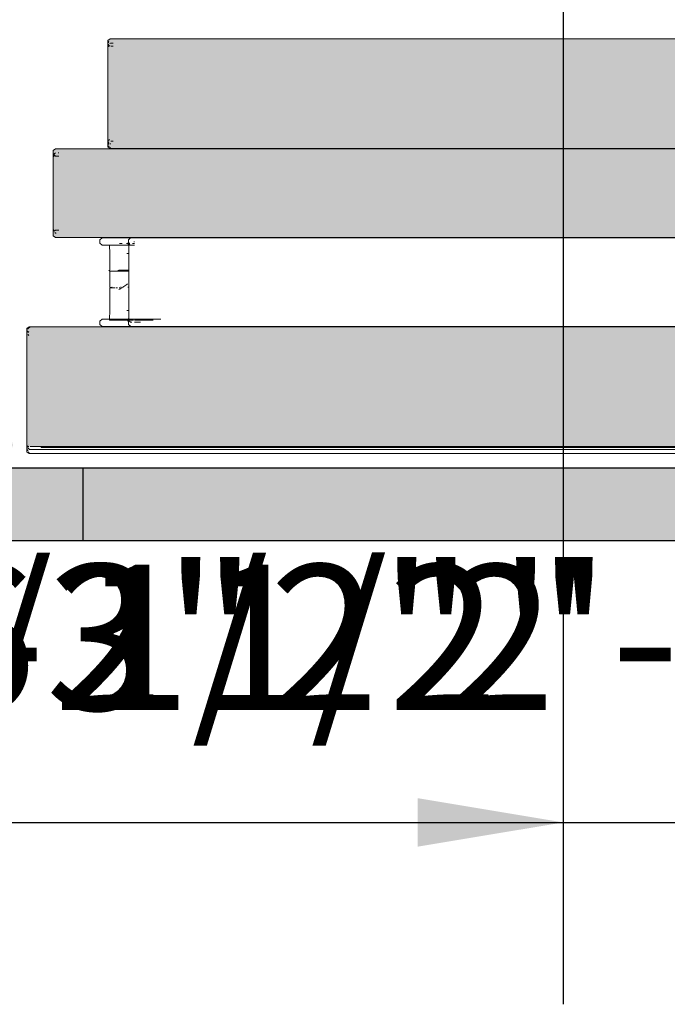
# Model space of a CAD drawing. Units: millimetres. Extents: x 7894 to 8038, y 6851 to 6951.
# Tile 17 of 49: x 7946.604 to 7951.055, y 6903.287 to 6910.053. Entities that reach past the tile are written whole.
import ezdxf

# ---------------------------------------------------------------- set-up
doc = ezdxf.new("R2010")
doc.units = ezdxf.units.MM
for name, color, linetype, lineweight in [('A-ANNO-DIMS', 2, 'Continuous', 18), ('A-FURN-BOOK', 8, 'Continuous', 13), ('A-FURN-SHLF', 7, 'Continuous', 30)]:
    doc.layers.add(name, color=color, linetype=linetype, lineweight=lineweight)
doc.layers.add('A-FURN-PATT', color=32, linetype='Continuous', lineweight=9, true_color=0xcd6928)
doc.styles.get("Standard").update_dxf_attribs({"font": 'arial.ttf'})
doc.dimstyles.new('ISO-25', dxfattribs={"dimtxt": 1, "dimasz": 1, "dimexe": 1.25, "dimexo": 0.625, "dimtad": 1, "dimdec": 0, "dimlunit": 4, "dimtxsty": 'Standard', "dimcen": 2.5, "dimclrt": 1, "dimadec": 0, "dimazin": 0, "dimtfac": 1, "dimtdec": 0, "dimtmove": 0, "dimatfit": 3, "dimfxl": 1, "dimarcsym": 0})

# ---------------------------------------------------------------- blocks, each defined once
blk = doc.blocks.new('*D23')
at = {"layer": 'A-ANNO-DIMS', "color": 0, "lineweight": -2, "transparency": 16777216}
for p, q in [((7940.0888, 6907.098), (7940.0888, 6947.7928)), ((7971.9356, 6928.989), (7971.9356, 6947.7928)), ((7941.0888, 6946.5428), (7970.9356, 6946.5428))]:
    blk.add_line(p, q, dxfattribs=at)
at = {"layer": 'A-ANNO-DIMS', "color": 0, "transparency": 16777216}
for points in [[(7941.0888, 6946.7095), (7941.0888, 6946.3762), (7940.0888, 6946.5428)], [(7970.9356, 6946.7095), (7970.9356, 6946.3762), (7971.9356, 6946.5428)]]:
    blk.add_solid(points, dxfattribs=at)
at = {"layer": 'Defpoints', "color": 0, "transparency": 16777216}
for p in [(7971.9356, 6946.5428), (7971.9356, 6928.364), (7940.0888, 6906.473)]:
    blk.add_point(p, dxfattribs=at)
at = {"layer": 'A-ANNO-DIMS', "color": 1, "transparency": 16777216, "insert": (7956.0122, 6947.6784), "char_height": 1, "attachment_point": 5}
blk.add_mtext('2\'-8"', dxfattribs=at)
blk = doc.blocks.new('*D24')
at = {"layer": 'A-ANNO-DIMS', "color": 0, "lineweight": -2, "transparency": 16777216}
for p, q in [((7953.3408, 6944.6059), (7936.9023, 6944.6059)), ((7938.1523, 6907.473), (7938.1523, 6943.6059)), ((7939.4638, 6906.473), (7936.9023, 6906.473))]:
    blk.add_line(p, q, dxfattribs=at)
at = {"layer": 'A-ANNO-DIMS', "color": 0, "transparency": 16777216}
for points in [[(7937.9856, 6943.6059), (7938.319, 6943.6059), (7938.1523, 6944.6059)], [(7937.9856, 6907.473), (7938.319, 6907.473), (7938.1523, 6906.473)]]:
    blk.add_solid(points, dxfattribs=at)
at = {"layer": 'Defpoints', "color": 0, "transparency": 16777216}
for p in [(7938.1523, 6944.6059), (7953.9658, 6944.6059), (7940.0888, 6906.473)]:
    blk.add_point(p, dxfattribs=at)
at = {"layer": 'A-ANNO-DIMS', "color": 1, "transparency": 16777216, "insert": (7937.0164, 6925.5395), "char_height": 1, "attachment_point": 5, "rotation": 90}
blk.add_mtext('3\'-2"', dxfattribs=at)
blk = doc.blocks.new('*D25')
at = {"layer": 'A-ANNO-DIMS', "color": 0, "lineweight": -2, "transparency": 16777216}
for p, q in [((7940.0888, 6905.848), (7940.0888, 6903.2865)), ((7964.3408, 6905.8484), (7964.3408, 6903.2865)), ((7941.0888, 6904.5365), (7963.3408, 6904.5365))]:
    blk.add_line(p, q, dxfattribs=at)
at = {"layer": 'A-ANNO-DIMS', "color": 0, "transparency": 16777216}
for points in [[(7941.0888, 6904.7032), (7941.0888, 6904.3699), (7940.0888, 6904.5365)], [(7963.3408, 6904.7032), (7963.3408, 6904.3699), (7964.3408, 6904.5365)]]:
    blk.add_solid(points, dxfattribs=at)
at = {"layer": 'Defpoints', "color": 0, "transparency": 16777216}
for p in [(7940.0888, 6906.473), (7964.3408, 6906.4734), (7964.3408, 6904.5365)]:
    blk.add_point(p, dxfattribs=at)
at = {"layer": 'A-ANNO-DIMS', "color": 1, "transparency": 16777216, "insert": (7952.2148, 6905.6786), "char_height": 1, "attachment_point": 5}
blk.add_mtext('2\'-0 1/2"', dxfattribs=at)
blk = doc.blocks.new('*D26')
at = {"layer": 'A-ANNO-DIMS', "color": 0, "lineweight": -2, "transparency": 16777216}
for p, q in [((7950.9654, 6918.7198), (7975.2272, 6918.7198)), ((7973.9772, 6917.7198), (7973.9772, 6907.4734)), ((7964.9658, 6906.4734), (7975.2272, 6906.4734))]:
    blk.add_line(p, q, dxfattribs=at)
at = {"layer": 'A-ANNO-DIMS', "color": 0, "transparency": 16777216}
for points in [[(7973.8105, 6917.7198), (7974.1439, 6917.7198), (7973.9772, 6918.7198)], [(7973.8105, 6907.4734), (7974.1439, 6907.4734), (7973.9772, 6906.4734)]]:
    blk.add_solid(points, dxfattribs=at)
at = {"layer": 'Defpoints', "color": 0, "transparency": 16777216}
for p in [(7950.3404, 6918.7198), (7964.3408, 6906.4734), (7973.9772, 6906.4734)]:
    blk.add_point(p, dxfattribs=at)
at = {"layer": 'A-ANNO-DIMS', "color": 1, "transparency": 16777216, "insert": (7972.8416, 6912.5966), "char_height": 1, "attachment_point": 5, "rotation": 90}
blk.add_mtext('1\'-0"', dxfattribs=at)
blk = doc.blocks.new('*D29')
at = {"layer": 'A-ANNO-DIMS', "color": 0, "lineweight": -2, "transparency": 16777216}
for p, q in [((7940.4346, 6923.8139), (7940.4346, 6903.2865)), ((7943.7365, 6918.0948), (7943.7365, 6903.2865)), ((7941.4346, 6904.5365), (7942.7365, 6904.5365)), ((7943.7365, 6904.5365), (7950.9749, 6904.5365))]:
    blk.add_line(p, q, dxfattribs=at)
at = {"layer": 'A-ANNO-DIMS', "color": 0, "transparency": 16777216}
for points in [[(7941.4346, 6904.7032), (7941.4346, 6904.3699), (7940.4346, 6904.5365)], [(7942.7365, 6904.7032), (7942.7365, 6904.3699), (7943.7365, 6904.5365)]]:
    blk.add_solid(points, dxfattribs=at)
at = {"layer": 'Defpoints', "color": 0, "transparency": 16777216}
for p in [(7940.4346, 6924.4389), (7943.7365, 6918.7198), (7943.7365, 6904.5365)]:
    blk.add_point(p, dxfattribs=at)
at = {"layer": 'A-ANNO-DIMS', "color": 1, "transparency": 16777216, "insert": (7947.8557, 6905.6789), "char_height": 1, "attachment_point": 5}
blk.add_mtext('0\'-3 1/2"', dxfattribs=at)
blk = doc.blocks.new('*D32')
at = {"layer": 'A-ANNO-DIMS', "color": 0, "lineweight": -2, "transparency": 16777216}
for p, q in [((7943.7365, 6918.0948), (7943.7365, 6903.2865)), ((7950.3404, 6918.0948), (7950.3404, 6903.2865)), ((7944.7365, 6904.5365), (7949.3404, 6904.5365))]:
    blk.add_line(p, q, dxfattribs=at)
at = {"layer": 'A-ANNO-DIMS', "color": 0, "transparency": 16777216}
for points in [[(7944.7365, 6904.7032), (7944.7365, 6904.3699), (7943.7365, 6904.5365)], [(7949.3404, 6904.7032), (7949.3404, 6904.3699), (7950.3404, 6904.5365)]]:
    blk.add_solid(points, dxfattribs=at)
at = {"layer": 'Defpoints', "color": 0, "transparency": 16777216}
for p in [(7943.7365, 6918.7198), (7950.3404, 6918.7198), (7950.3404, 6904.5365)]:
    blk.add_point(p, dxfattribs=at)
at = {"layer": 'A-ANNO-DIMS', "color": 1, "transparency": 16777216, "insert": (7947.0385, 6905.6786), "char_height": 1, "attachment_point": 5}
blk.add_mtext('0\'-6 1/2"', dxfattribs=at)
blk = doc.blocks.new('*D33')
at = {"layer": 'A-ANNO-DIMS', "color": 0, "lineweight": -2, "transparency": 16777216}
for p, q in [((7940.4346, 6923.8139), (7940.4346, 6903.2865)), ((7940.0888, 6905.848), (7940.0888, 6903.2865)), ((7939.0888, 6904.5365), (7938.0888, 6904.5365)), ((7940.0888, 6904.5365), (7940.4346, 6904.5365)), ((7941.4346, 6904.5365), (7948.673, 6904.5365))]:
    blk.add_line(p, q, dxfattribs=at)
at = {"layer": 'A-ANNO-DIMS', "color": 0, "transparency": 16777216}
for points in [[(7939.0888, 6904.7032), (7939.0888, 6904.3699), (7940.0888, 6904.5365)], [(7941.4346, 6904.7032), (7941.4346, 6904.3699), (7940.4346, 6904.5365)]]:
    blk.add_solid(points, dxfattribs=at)
at = {"layer": 'Defpoints', "color": 0, "transparency": 16777216}
for p in [(7940.4346, 6924.4389), (7940.0888, 6906.473), (7940.4346, 6904.5365)]:
    blk.add_point(p, dxfattribs=at)
at = {"layer": 'A-ANNO-DIMS', "color": 1, "transparency": 16777216, "insert": (7945.5538, 6905.6786), "char_height": 1, "attachment_point": 5}
blk.add_mtext('0\'-0 1/2"', dxfattribs=at)

msp = doc.modelspace()

# ---------------------------------------------------------------- hatches: boundary and pattern name
at = {"layer": 'A-FURN-PATT'}
h = msp.add_hatch(color=256, dxfattribs=at)
h.dxf.hatch_style = 1
h.paths.add_polyline_path([(7942.8406, 6913.3629), (7942.8593, 6913.356), (7942.8677, 6913.356), (7942.8677, 6914.2132), (7942.876, 6914.2376), (7942.8813, 6914.2376), (7942.9022, 6914.2457), (7943.3657, 6914.2457), (7943.3844, 6914.2376), (7943.3861, 6914.2376), (7943.3858, 6914.2132), (7943.3852, 6913.2312), (7943.3944, 6906.9948), (7943.387, 6906.9732), (7943.4027, 6906.9732), (7943.403, 6906.9948), (7943.4029, 6908.4372), (7943.3944, 6914.2132), (7943.4169, 6914.2376), (7943.4198, 6914.2457), (7943.4555, 6914.2457), (7943.4603, 6914.238), (7943.8607, 6914.2452), (7943.8615, 6914.2457), (7943.8623, 6914.2452), (7943.8866, 6914.2457), (7943.8944, 6914.2402), (7943.9104, 6914.2376), (7943.9211, 6914.2132), (7943.9294, 6914.2376), (7943.9318, 6914.2376), (7943.9453, 6914.2398), (7943.9488, 6914.2457), (7943.9797, 6914.2452), (7943.9807, 6914.2457), (7943.9815, 6914.2451), (7944.3738, 6914.2376), (7944.3882, 6914.2457), (7944.4201, 6914.2457), (7944.4341, 6914.2376), (7944.4395, 6914.2376), (7944.4478, 6914.2132), (7944.4478, 6914.1031), (7944.4622, 6914.099), (7944.7359, 6914.1607), (7944.8923, 6914.2014), (7944.9541, 6914.2098), (7944.955, 6914.21), (7946.556, 6907.1325), (7946.5534, 6907.1122), (7946.5529, 6907.1152), (7946.499, 6907.103), (7946.3343, 6907.0604), (7946.0282, 6906.9914), (7945.6731, 6908.5712), (7944.4484, 6914.0015), (7944.4478, 6906.9948), (7944.4404, 6906.9732), (7947.0373, 6906.9734), (7964.3408, 6906.9734), (7964.3408, 6906.4734), (7947.0373, 6906.4734), (7940.0888, 6906.473), (7940.0888, 6906.973), (7941.9951, 6906.9731), (7941.9899, 6906.9898), (7941.9899, 6913.3353), (7941.9968, 6913.3574), (7942.003, 6913.3571), (7942.0169, 6913.3629), (7942.0366, 6913.3629), (7942.0378, 6913.3629), (7942.0479, 6913.356), (7942.8142, 6913.356), (7942.8157, 6913.356), (7942.8346, 6913.356)])
h.paths.add_polyline_path([(7942.8598, 6913.0201), (7942.861, 6913.3353), (7942.8677, 6906.9948), (7942.876, 6906.9759), (7942.876, 6906.9903), (7942.8813, 6914.2376), (7942.876, 6914.2321), (7942.876, 6914.2177), (7942.8809, 6906.9647), (7942.8784, 6906.9704), (7942.876, 6906.9704), (7942.8574, 6906.9704), (7942.8613, 6911.8549)], flags=16)
h.paths.add_polyline_path([(7942.8613, 6911.8549), (7942.8677, 6906.9948), (7942.8686, 6906.9921), (7942.8677, 6906.9898), (7942.8616, 6906.9704), (7942.8598, 6906.9704), (7942.8574, 6906.9704), (7942.0002, 6906.9704), (7941.9978, 6906.9704), (7941.996, 6906.9704), (7941.9899, 6906.9898), (7941.9978, 6906.9704), (7942.0002, 6906.9704), (7942.8598, 6906.9704), (7942.8616, 6906.9748)], flags=16)
h.paths.add_polyline_path([(7942.023, 6913.356), (7942.0169, 6913.3629), (7942.0366, 6913.3629), (7942.0378, 6913.3629), (7942.0367, 6913.3614), (7942.0369, 6913.356)], flags=16)
h.paths.add_polyline_path([(7942.0366, 6913.3629), (7942.0169, 6913.3629), (7942.0196, 6913.3598)], flags=0)
h.paths.add_polyline_path([(7942.0353, 6913.356), (7942.0369, 6913.356), (7942.0367, 6913.3614)], flags=0)
h.paths.add_polyline_path([(7943.9293, 6906.9759), (7943.9211, 6906.9948), (7943.9294, 6906.9704)], flags=0)
h.paths.add_polyline_path([(7943.9125, 6914.2132), (7943.8982, 6914.2376), (7943.8944, 6914.2402), (7943.8832, 6914.2421), (7943.8781, 6914.2367), (7943.8765, 6914.2376), (7943.8789, 6914.2376), (7943.8866, 6914.2457), (7943.8623, 6914.2452), (7943.8607, 6914.2452), (7943.8615, 6914.2457), (7943.8623, 6914.2452), (7943.8866, 6914.2457), (7943.8944, 6914.2402), (7943.8982, 6914.2376), (7943.9097, 6914.218), (7943.9125, 6914.2168), (7943.9079, 6906.9704), (7943.9104, 6906.9704), (7943.9211, 6914.2132), (7943.9294, 6914.2376), (7943.9318, 6914.2376), (7943.9453, 6914.2398), (7943.9488, 6914.2457), (7943.9797, 6914.2452), (7943.9807, 6914.2457), (7943.9815, 6914.2451), (7944.3738, 6914.2376), (7944.3882, 6914.2457), (7944.4201, 6914.2457), (7944.4341, 6914.2376), (7944.4395, 6914.2376), (7944.4395, 6914.2177), (7944.4341, 6914.0941), (7944.4478, 6914.1004), (7944.4513, 6914.1021), (7944.4622, 6914.099), (7944.4343, 6914.0927), (7944.429, 6914.0915), (7944.4341, 6914.069), (7944.4484, 6914.0015), (7944.4341, 6914.0649), (7944.4346, 6906.9704), (7944.4371, 6906.9704), (7944.4395, 6906.9759), (7944.4395, 6906.9704), (7943.931, 6906.9704), (7943.9128, 6906.9704), (7943.9079, 6906.9704)], flags=16)
h.paths.add_polyline_path([(7943.9211, 6914.2132), (7943.9294, 6914.2376), (7943.9318, 6914.2376), (7943.9453, 6914.2398), (7943.9488, 6914.2457), (7943.9797, 6914.2452), (7943.9807, 6914.2457), (7943.9815, 6914.2451), (7944.3738, 6914.2376), (7944.3882, 6914.2457), (7944.4201, 6914.2457), (7944.4321, 6914.2387), (7944.4249, 6914.2376), (7944.4041, 6914.2376), (7944.4032, 6914.2136), (7944.4032, 6914.2376), (7944.4025, 6914.2379), (7944.3897, 6914.2382), (7944.3753, 6914.2384), (7944.3738, 6914.2376), (7943.9815, 6914.2451), (7943.9488, 6914.2457), (7943.9453, 6914.2398), (7943.9294, 6914.2132), (7943.931, 6906.9721), (7943.931, 6906.9704), (7943.9294, 6906.9704), (7943.9293, 6906.9759), (7943.9294, 6914.2132), (7943.9439, 6914.2376), (7943.9318, 6914.2376)], flags=0)
h.paths.add_polyline_path([(7942.8813, 6914.2376), (7942.8778, 6914.2362), (7942.8796, 6914.2404), (7942.885, 6914.239)], flags=17)
h.paths.add_polyline_path([(7944.4116, 6914.242), (7944.4104, 6914.2408), (7944.4125, 6914.2418)], flags=0)
h.paths.add_polyline_path([(7944.3879, 6914.2382), (7944.3882, 6914.2457), (7944.4094, 6914.241), (7944.4103, 6914.2408), (7944.4036, 6914.2373), (7944.39, 6914.2447), (7944.3897, 6914.2382)], flags=0)
h.paths.add_polyline_path([(7963.1359, 6906.9526), (7963.1396, 6906.9526), (7963.1431, 6906.9582)], flags=16)
h.paths.add_polyline_path([(7954.3975, 6907.3902), (7954.397, 6907.3948), (7954.3984, 6907.4007), (7954.3975, 6907.567), (7954.3984, 6907.5978), (7954.3986, 6907.7694), (7954.3978, 6907.7989), (7954.399, 6907.8759), (7954.3992, 6907.9037), (7954.3944, 6907.9081), (7954.4019, 6907.9055), (7954.3996, 6907.93), (7954.3988, 6907.9307), (7954.3841, 6907.9429), (7946.6754, 6907.9429), (7946.6535, 6907.9232), (7946.6531, 6907.9127), (7946.6527, 6907.7694), (7946.6525, 6907.4007), (7946.653, 6907.1185), (7946.6574, 6907.1224), (7946.656, 6907.1145), (7946.6571, 6907.1135), (7946.6675, 6907.1209), (7946.7515, 6907.1209), (7946.9105, 6907.1209), (7954.3003, 6907.1209), (7954.3895, 6907.1209), (7954.3915, 6907.1191), (7954.3991, 6907.1209), (7954.399, 6907.1383), (7954.3978, 6907.2163), (7954.3986, 6907.2413)], flags=17)
h.paths.add_polyline_path([(7954.3003, 6907.1209), (7954.3003, 6907.1136), (7946.9105, 6907.1129), (7946.7516, 6907.1136), (7946.7515, 6907.1209), (7946.6675, 6907.1209), (7946.6531, 6907.1106), (7946.653, 6907.1185), (7946.6574, 6907.1224), (7946.656, 6907.1145), (7946.6571, 6907.1135), (7946.6675, 6907.1209), (7946.7515, 6907.1209), (7946.9105, 6907.1209)], flags=17)
h.paths.add_polyline_path([(7954.3981, 6907.9048), (7954.3944, 6907.9081), (7954.3997, 6907.9062), (7954.4007, 6907.9186), (7954.4019, 6907.9055), (7954.405, 6907.9072), (7954.4044, 6907.9046), (7954.4027, 6907.8974), (7954.4024, 6907.9009), (7954.3996, 6907.9034), (7954.3996, 6907.9025), (7954.3994, 6907.9023), (7954.3995, 6907.9035)], flags=17)
h = msp.add_hatch(color=256, dxfattribs=at)
h.dxf.hatch_style = 1
h.paths.add_polyline_path([(7954.384, 6909.6263), (7954.383, 6909.6719), (7954.3832, 6909.6719), (7954.3841, 6909.7804), (7954.3842, 6909.8528), (7954.3843, 6909.8691), (7954.3797, 6909.8762), (7954.3846, 6909.8799), (7954.3847, 6909.8812), (7954.3833, 6909.8825), (7954.3848, 6909.8826), (7954.3858, 6909.8967), (7954.3849, 6909.9082), (7954.384, 6909.909), (7954.384, 6909.9101), (7954.3682, 6909.9217), (7947.2251, 6909.9217), (7947.21, 6909.9101), (7947.2092, 6909.8906), (7947.2092, 6909.1993), (7947.2105, 6909.1985), (7947.2109, 6909.2125), (7947.2127, 6909.2113), (7947.2135, 6909.2114), (7947.2139, 6909.2117), (7947.2148, 6909.196), (7947.2105, 6909.1985), (7947.21, 6909.1798), (7947.2251, 6909.1682), (7947.2316, 6909.1682), (7954.3693, 6909.1682), (7954.384, 6909.1798), (7954.385, 6909.1814), (7954.3858, 6909.1921), (7954.3871, 6909.207), (7954.3814, 6909.2115), (7954.377, 6909.2116), (7954.3506, 6909.2116), (7954.3427, 6909.2213), (7954.373, 6909.2213), (7954.3747, 6909.2192), (7954.3833, 6909.2192), (7954.3833, 6909.2247), (7954.3843, 6909.2237), (7954.3842, 6909.2371), (7954.384, 6909.4541), (7954.3827, 6909.477), (7954.3832, 6909.477)])
h.paths.add_polyline_path([(7947.2139, 6909.8782), (7947.214, 6909.8795), (7947.2135, 6909.8785)], flags=16)
h.paths.add_polyline_path([(7947.2105, 6909.1985), (7947.2109, 6909.2125), (7947.2127, 6909.2113), (7947.2135, 6909.2114), (7947.2139, 6909.2117), (7947.2144, 6909.2034), (7947.2148, 6909.196)], flags=17)
h.paths.add_polyline_path([(7954.3858, 6909.1921), (7954.3848, 6909.2088), (7954.3871, 6909.207)], flags=17)
h.paths.add_polyline_path([(7954.5846, 6909.1237), (7954.5837, 6909.1245), (7954.5808, 6909.1271), (7954.5846, 6909.1307), (7954.5846, 6909.1519), (7954.5691, 6909.1658), (7946.8503, 6909.1658), (7946.8349, 6909.1546), (7946.8349, 6909.1307), (7946.8349, 6909.1147), (7946.8349, 6909.1147), (7946.8349, 6908.5685), (7946.8503, 6908.5572), (7954.5691, 6908.5572), (7954.5846, 6908.5685)])
h.paths.add_polyline_path([(7946.8375, 6909.1282), (7946.8349, 6909.1263), (7946.8349, 6909.1237), (7946.8473, 6909.1162), (7946.8503, 6909.1162)], flags=16)

# ---------------------------------------------------------------- linework, layer by layer
at = {"layer": 'A-FURN-BOOK'}
for p, q in [((7947.2092, 6909.8906), (7947.21, 6909.9101)), ((7947.2092, 6909.8906), (7947.2092, 6909.1993)), ((7947.21, 6909.9101), (7947.2251, 6909.9217)), ((7947.21, 6909.9101), (7947.2105, 6909.8913)), ((7947.2106, 6909.8888), (7947.2113, 6909.8799)), ((7947.2119, 6909.8784), (7947.2113, 6909.8799)), ((7947.2119, 6909.8784), (7947.2135, 6909.8785)), ((7947.2131, 6909.8717), (7947.2119, 6909.8784)), ((7947.2135, 6909.8785), (7947.214, 6909.8795)), ((7947.2135, 6909.8785), (7947.2227, 6909.8701)), ((7947.214, 6909.8795), (7947.2142, 6909.8839)), ((7947.2164, 6909.8811), (7947.214, 6909.8795)), ((7947.2148, 6909.8938), (7947.2153, 6909.901)), ((7947.2153, 6909.901), (7947.2159, 6909.9056)), ((7947.229, 6909.8928), (7947.2242, 6909.8884)), ((7954.3693, 6909.9217), (7947.2251, 6909.9217)), ((7947.2472, 6909.8928), (7947.229, 6909.8928)), ((7947.2135, 6909.8692), (7947.2131, 6909.8717)), ((7947.2156, 6909.8672), (7947.2135, 6909.8692)), ((7947.2242, 6909.8703), (7947.2227, 6909.8701)), ((7947.2316, 6909.8707), (7947.2471, 6909.8707)), ((7947.2105, 6909.1985), (7947.2092, 6909.1993)), ((7947.21, 6909.1798), (7947.2105, 6909.1985)), ((7947.2105, 6909.1985), (7947.2108, 6909.2098)), ((7947.2108, 6909.2098), (7947.2114, 6909.2111)), ((7947.2114, 6909.2111), (7947.212, 6909.2127)), ((7947.2135, 6909.2114), (7947.2114, 6909.2111)), ((7947.212, 6909.2127), (7947.2128, 6909.217)), ((7947.2147, 6909.2126), (7947.2135, 6909.2114)), ((7947.214, 6909.2104), (7947.2135, 6909.2114)), ((7947.2144, 6909.2034), (7947.214, 6909.2104)), ((7947.2164, 6909.2087), (7947.214, 6909.2104)), ((7947.2148, 6909.196), (7947.2144, 6909.2034)), ((7947.2226, 6909.2291), (7947.2156, 6909.2227)), ((7947.229, 6909.1971), (7947.2242, 6909.2015)), ((7947.2471, 6909.2192), (7947.2316, 6909.2192)), ((7946.8349, 6909.1546), (7946.8503, 6909.1658)), ((7946.8349, 6909.1307), (7946.8349, 6909.1546)), ((7946.8503, 6909.1377), (7946.8349, 6909.1263)), ((7946.8349, 6909.1263), (7946.8349, 6909.1307)), ((7946.8503, 6909.1162), (7946.8349, 6909.1307)), ((7954.5691, 6909.1658), (7946.8503, 6909.1658)), ((7946.8732, 6909.1377), (7946.868, 6909.1377)), ((7947.2251, 6909.1682), (7947.21, 6909.1798)), ((7947.2161, 6909.1825), (7947.2155, 6909.1869)), ((7947.2193, 6909.1795), (7947.2161, 6909.1825)), ((7947.2316, 6909.1682), (7947.2249, 6909.1744)), ((7947.2251, 6909.1682), (7947.2316, 6909.1682)), ((7947.2316, 6909.1682), (7954.3693, 6909.1682)), ((7946.8349, 6909.1237), (7946.8349, 6909.1263)), ((7946.8484, 6909.1155), (7946.8349, 6909.1237)), ((7946.8349, 6909.1147), (7946.8349, 6909.1237)), ((7946.8383, 6909.1116), (7946.8349, 6909.1147)), ((7946.8349, 6908.5685), (7946.8349, 6909.1147)), ((7946.8732, 6909.1162), (7946.8503, 6909.1162)), ((7946.8383, 6908.6114), (7946.8363, 6908.6096)), ((7946.8484, 6908.6075), (7946.84, 6908.6014)), ((7946.8413, 6908.5987), (7946.8503, 6908.6068)), ((7946.8503, 6908.5853), (7946.8454, 6908.5898)), ((7946.8503, 6908.6068), (7946.8732, 6908.6068)), ((7946.8503, 6908.5572), (7946.8349, 6908.5685)), ((7946.8555, 6908.5853), (7946.8503, 6908.5853)), ((7954.5691, 6908.5572), (7946.8503, 6908.5572)), ((7947.1561, 6908.5403), (7947.1715, 6908.5542)), ((7947.1561, 6908.5185), (7947.1561, 6908.5403)), ((7947.3682, 6908.5542), (7947.1715, 6908.5542)), ((7947.3517, 6908.5299), (7947.3504, 6908.5168)), ((7947.3526, 6908.5411), (7947.3517, 6908.5299)), ((7947.3517, 6908.5299), (7947.3528, 6908.516)), ((7947.3535, 6908.543), (7947.3526, 6908.5411)), ((7947.3536, 6908.5419), (7947.3526, 6908.5411)), ((7947.3535, 6908.543), (7947.3623, 6908.5492)), ((7947.3623, 6908.5492), (7947.3543, 6908.5425)), ((7947.3682, 6908.5542), (7947.3623, 6908.5492)), ((7947.3682, 6908.5542), (7954.5763, 6908.5542)), ((7947.3931, 6908.5261), (7947.3883, 6908.5261)), ((7947.1715, 6908.5046), (7947.1561, 6908.5185)), ((7947.1715, 6908.5046), (7947.2224, 6908.5046)), ((7947.223, 6908.4455), (7947.2224, 6908.5046)), ((7947.344, 6908.5046), (7947.2224, 6908.5046)), ((7947.2904, 6908.516), (7947.2891, 6908.5158)), ((7947.2904, 6908.516), (7947.3087, 6908.5158)), ((7947.3387, 6908.516), (7947.3479, 6908.516)), ((7947.344, 6908.5046), (7947.3495, 6908.5038)), ((7947.3474, 6908.5185), (7947.3479, 6908.516)), ((7947.3504, 6908.5168), (7947.3474, 6908.5185)), ((7947.3479, 6908.516), (7947.3504, 6908.5168)), ((7947.3479, 6908.516), (7947.3482, 6908.5147)), ((7947.3482, 6908.5147), (7947.3491, 6908.5074)), ((7947.3491, 6908.5074), (7947.3495, 6908.5038)), ((7947.3495, 6908.5038), (7947.35, 6908.5031)), ((7947.3495, 6908.5038), (7947.3532, 6908.5031)), ((7947.3504, 6908.5168), (7947.35, 6908.5122)), ((7947.3527, 6908.5138), (7947.35, 6908.5122)), ((7947.3533, 6908.5002), (7947.35, 6908.5031)), ((7947.3504, 6908.5168), (7947.3528, 6908.516)), ((7947.3542, 6908.516), (7947.3527, 6908.5147)), ((7947.3528, 6908.516), (7947.3527, 6908.5147)), ((7947.3527, 6908.5147), (7947.3527, 6908.5138)), ((7947.365, 6908.5046), (7947.3527, 6908.5138)), ((7947.3628, 6908.5046), (7947.3527, 6908.5138)), ((7947.3527, 6908.5138), (7947.3532, 6908.5031)), ((7947.3528, 6908.516), (7947.3542, 6908.516)), ((7947.3579, 6908.5046), (7947.3532, 6908.5031)), ((7947.3532, 6908.5031), (7947.3668, 6908.5033)), ((7947.3532, 6908.5031), (7947.3533, 6908.5002)), ((7947.3533, 6908.5002), (7947.3534, 6908.4872)), ((7947.3547, 6908.4988), (7947.3533, 6908.5002)), ((7947.3534, 6908.4872), (7947.3546, 6908.4455)), ((7947.358, 6908.5195), (7947.3542, 6908.516)), ((7947.3542, 6908.516), (7947.3608, 6908.516)), ((7947.3628, 6908.5046), (7947.3579, 6908.5046)), ((7947.365, 6908.5046), (7947.3628, 6908.5046)), ((7947.3668, 6908.5033), (7947.365, 6908.5046)), ((7947.3703, 6908.5046), (7947.365, 6908.5046)), ((7947.3668, 6908.5033), (7947.3703, 6908.5046)), ((7947.3932, 6908.5046), (7947.3703, 6908.5046)), ((7947.3797, 6908.516), (7947.3931, 6908.516)), ((7947.2236, 6908.3704), (7947.223, 6908.4455)), ((7947.3546, 6908.4455), (7947.3402, 6908.4455)), ((7947.3546, 6908.4455), (7947.3538, 6908.4287)), ((7947.3538, 6908.4287), (7947.3539, 6908.3323)), ((7947.2237, 6908.3323), (7947.2168, 6908.3291)), ((7947.2238, 6908.3258), (7947.2168, 6908.3291)), ((7947.2236, 6908.3704), (7947.2237, 6908.3323)), ((7947.2239, 6908.2877), (7947.2238, 6908.3258)), ((7947.2238, 6908.3258), (7947.3539, 6908.3258)), ((7947.2778, 6908.3291), (7947.2844, 6908.3291)), ((7947.3539, 6908.3323), (7947.285, 6908.3323)), ((7947.3275, 6908.3291), (7947.3539, 6908.3291)), ((7947.3548, 6908.3323), (7947.3539, 6908.3323)), ((7947.3539, 6908.3323), (7947.3539, 6908.3291)), ((7947.3539, 6908.3291), (7947.3548, 6908.3291)), ((7947.3539, 6908.3291), (7947.3539, 6908.3258)), ((7947.3539, 6908.3258), (7947.3548, 6908.3258)), ((7947.3539, 6908.3258), (7947.354, 6908.3136)), ((7947.2239, 6908.2877), (7947.2239, 6908.2159)), ((7947.354, 6908.3136), (7947.354, 6908.2159)), ((7947.2239, 6908.2093), (7947.2236, 6908.1299)), ((7947.2346, 6908.2126), (7947.2239, 6908.2159)), ((7947.2239, 6908.2093), (7947.2346, 6908.2126)), ((7947.2586, 6908.2093), (7947.2239, 6908.2093)), ((7947.2372, 6908.2159), (7947.2409, 6908.2159)), ((7947.2756, 6908.2093), (7947.2643, 6908.2093)), ((7947.2846, 6908.1978), (7947.2926, 6908.2011)), ((7947.2921, 6908.2093), (7947.2872, 6908.2093)), ((7947.3045, 6908.2093), (7947.2926, 6908.2011)), ((7947.2972, 6908.2159), (7947.3021, 6908.2159)), ((7947.3045, 6908.2093), (7947.314, 6908.2159)), ((7947.3075, 6908.2093), (7947.3045, 6908.2093)), ((7947.314, 6908.2159), (7947.3395, 6908.2338)), ((7947.314, 6908.2159), (7947.3175, 6908.2159)), ((7947.3448, 6908.2371), (7947.3395, 6908.2338)), ((7947.3478, 6908.2159), (7947.354, 6908.2159)), ((7947.354, 6908.2093), (7947.3516, 6908.2093)), ((7947.354, 6908.1815), (7947.3538, 6908.0745)), ((7947.354, 6908.2159), (7947.3548, 6908.2159)), ((7947.354, 6908.2159), (7947.354, 6908.2093)), ((7947.3548, 6908.2093), (7947.354, 6908.2093)), ((7947.354, 6908.2093), (7947.354, 6908.1815)), ((7947.223, 6908.0548), (7947.2236, 6908.1299)), ((7947.2224, 6907.9952), (7947.223, 6908.0548)), ((7947.3403, 6908.0548), (7947.3537, 6908.0548)), ((7947.3537, 6908.0548), (7947.3535, 6908.0126)), ((7947.3538, 6908.0745), (7947.3537, 6908.0548)), ((7947.3537, 6908.0548), (7947.3546, 6908.0548)), ((7947.1561, 6907.9813), (7947.1715, 6907.9952)), ((7947.1561, 6907.9595), (7947.1561, 6907.9813)), ((7947.2224, 6907.9952), (7947.1715, 6907.9952)), ((7947.2223, 6907.9873), (7947.2224, 6907.9952)), ((7947.2223, 6907.9873), (7947.3485, 6907.9877)), ((7947.2224, 6907.9952), (7947.3211, 6907.9952)), ((7947.3495, 6907.9961), (7947.3211, 6907.9952)), ((7947.3482, 6907.9851), (7947.3474, 6907.9813)), ((7947.3474, 6907.9813), (7947.3504, 6907.9834)), ((7947.3485, 6907.9877), (7947.3482, 6907.9851)), ((7947.3491, 6907.9923), (7947.3485, 6907.9877)), ((7947.3485, 6907.9877), (7947.35, 6907.9876)), ((7947.3495, 6907.9961), (7947.3491, 6907.9923)), ((7947.35, 6907.9967), (7947.3495, 6907.9961)), ((7947.3532, 6907.9952), (7947.3495, 6907.9961)), ((7947.3533, 6907.9997), (7947.35, 6907.9967)), ((7947.35, 6907.9876), (7947.3528, 6907.9877)), ((7947.35, 6907.9876), (7947.3504, 6907.9834)), ((7947.3527, 6907.9851), (7947.35, 6907.9876)), ((7947.3504, 6907.9834), (7947.3527, 6907.9851)), ((7947.3504, 6907.9834), (7947.3517, 6907.9689)), ((7947.3517, 6907.9689), (7947.3527, 6907.9851)), ((7947.3528, 6907.9877), (7947.3527, 6907.9861)), ((7947.3527, 6907.9851), (7947.3527, 6907.9861)), ((7947.3654, 6907.9737), (7947.3527, 6907.9851)), ((7947.3532, 6907.9952), (7947.3528, 6907.9877)), ((7947.3544, 6907.9877), (7947.3528, 6907.9877)), ((7947.3533, 6907.9997), (7947.3532, 6907.9967)), ((7947.3532, 6907.9967), (7947.3532, 6907.9952)), ((7947.3532, 6907.9952), (7947.3628, 6907.9952)), ((7947.3535, 6908.0126), (7947.3533, 6907.9997)), ((7947.3547, 6908.001), (7947.3533, 6907.9997)), ((7947.365, 6907.9952), (7947.3544, 6907.9877)), ((7947.3544, 6907.9877), (7947.3628, 6907.9952)), ((7947.3544, 6907.9877), (7947.3871, 6907.9878)), ((7947.3628, 6907.9952), (7947.365, 6907.9952)), ((7947.3668, 6907.9965), (7947.365, 6907.9952)), ((7947.365, 6907.9952), (7947.4524, 6907.9952)), ((7947.3932, 6907.9873), (7947.4524, 6907.988)), ((7947.4524, 6907.988), (7947.4524, 6907.9952)), ((7947.5742, 6907.9952), (7947.4524, 6907.9952)), ((7947.5222, 6907.9873), (7947.4524, 6907.988)), ((7946.6531, 6907.9127), (7946.6527, 6907.7694)), ((7946.6531, 6907.9127), (7946.6538, 6907.9317)), ((7946.6538, 6907.9317), (7946.669, 6907.9429)), ((7946.6543, 6907.9134), (7946.6544, 6907.911)), ((7946.6582, 6907.9078), (7946.6587, 6907.9158)), ((7946.6597, 6907.9273), (7946.66, 6907.929)), ((7946.66, 6907.929), (7946.6754, 6907.9429)), ((7946.669, 6907.9429), (7946.6754, 6907.9429)), ((7946.6754, 6907.9429), (7954.3841, 6907.9429)), ((7947.1715, 6907.9456), (7947.1561, 6907.9595)), ((7947.1715, 6907.9456), (7947.3682, 6907.9456)), ((7947.3517, 6907.9689), (7947.3526, 6907.9584)), ((7947.3526, 6907.9584), (7947.3535, 6907.9569)), ((7947.3682, 6907.9456), (7947.3535, 6907.9569)), ((7947.3754, 6907.9737), (7947.3654, 6907.9737)), ((7954.5828, 6907.9456), (7947.3682, 6907.9456)), ((7947.4341, 6907.9737), (7947.3931, 6907.9737)), ((7946.6581, 6907.9062), (7946.6582, 6907.9078)), ((7946.668, 6907.8823), (7946.6595, 6907.8899)), ((7946.6681, 6907.9105), (7946.6602, 6907.9034)), ((7946.6665, 6907.8927), (7946.668, 6907.8915)), ((7946.6527, 6907.7694), (7946.6525, 6907.4007)), ((7946.6525, 6907.4007), (7946.6531, 6907.1015)), ((7946.6543, 6907.1008), (7946.6531, 6907.1015)), ((7946.6543, 6907.1008), (7946.6538, 6907.0825)), ((7946.6567, 6907.1186), (7946.6569, 6907.1199)), ((7946.6569, 6907.1199), (7946.6574, 6907.1224)), ((7946.6595, 6907.1242), (7946.6574, 6907.1224)), ((7946.6681, 6907.1213), (7946.6585, 6907.1145)), ((7946.6728, 6907.0994), (7946.6602, 6907.1107)), ((7946.668, 6907.1319), (7946.6667, 6907.1308)), ((7954.3822, 6907.0994), (7946.6728, 6907.0994)), ((7946.7515, 6907.1209), (7946.6754, 6907.1209)), ((7946.7516, 6907.1136), (7946.7515, 6907.1209)), ((7946.7515, 6907.1209), (7946.9105, 6907.1209)), ((7946.9105, 6907.1129), (7946.7516, 6907.1136)), ((7946.9105, 6907.1129), (7946.9105, 6907.1209)), ((7954.3003, 6907.1209), (7946.9105, 6907.1209)), ((7954.3003, 6907.1136), (7946.9105, 6907.1129)), ((7946.669, 6907.0713), (7946.6538, 6907.0825)), ((7946.6591, 6907.0914), (7946.6587, 6907.0984)), ((7946.6594, 6907.0895), (7946.6591, 6907.0914)), ((7946.6687, 6907.0773), (7946.6632, 6907.0823)), ((7954.3841, 6907.0713), (7946.669, 6907.0713))]:
    msp.add_line(p, q, dxfattribs=at)
at = {"layer": 'A-FURN-SHLF'}
for p, q in [((7940.0888, 6906.973), (7947.0373, 6906.9734)), ((7947.0373, 6906.9734), (7964.3408, 6906.9734)), ((7947.0373, 6906.9734), (7947.0373, 6906.4734)), ((7940.0888, 6906.473), (7947.0373, 6906.4734)), ((7947.0373, 6906.4734), (7964.3408, 6906.4734))]:
    msp.add_line(p, q, dxfattribs=at)

# ---------------------------------------------------------------- dimensions: what is measured, and where the dimension line sits
at = {"layer": 'A-ANNO-DIMS'}
for base, p1, p2, picture, middle in [((7971.9356, 6946.5428), (7940.0888, 6906.473), (7971.9356, 6928.364), '*D23', (7956.0122, 6947.6784)), ((7940.4346, 6904.5365), (7940.0888, 6906.473), (7940.4346, 6924.4389), '*D33', (7945.5538, 6905.6786)), ((7943.7365, 6904.5365), (7940.4346, 6924.4389), (7943.7365, 6918.7198), '*D29', (7947.8557, 6905.6789)), ((7950.3404, 6904.5365), (7943.7365, 6918.7198), (7950.3404, 6918.7198), '*D32', (7947.0385, 6905.6786)), ((7964.3408, 6904.5365), (7940.0888, 6906.473), (7964.3408, 6906.4734), '*D25', (7952.2148, 6905.6786))]:
    dim = msp.add_linear_dim(base=base, p1=p1, p2=p2, dimstyle='ISO-25', override={"dimdec": 1, "dimlfac": 1, "dimrnd": 0, "dimzin": 1, "dimdsep": 46, "dimlunit": 4, "dimfrac": 2}, dxfattribs=at)
    dim.commit()
    dim.dimension.update_dxf_attribs({"geometry": picture, "text_midpoint": middle})
for base, p1, p2, picture, middle in [((7938.1523, 6944.6059), (7940.0888, 6906.473), (7953.9658, 6944.6059), '*D24', (7937.0164, 6925.5395)), ((7973.9772, 6906.4734), (7950.3404, 6918.7198), (7964.3408, 6906.4734), '*D26', (7972.8416, 6912.5966))]:
    dim = msp.add_linear_dim(base=base, p1=p1, p2=p2, angle=90, dimstyle='ISO-25', override={"dimdec": 1, "dimlfac": 1, "dimrnd": 0, "dimzin": 1, "dimdsep": 46, "dimlunit": 4, "dimfrac": 2}, dxfattribs=at)
    dim.commit()
    dim.dimension.update_dxf_attribs({"geometry": picture, "text_midpoint": middle})

doc.saveas('drawing.dxf')
